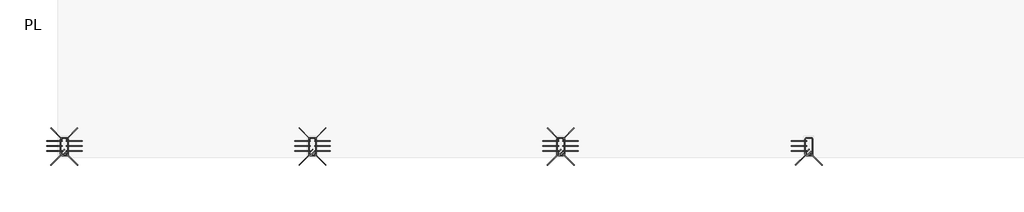
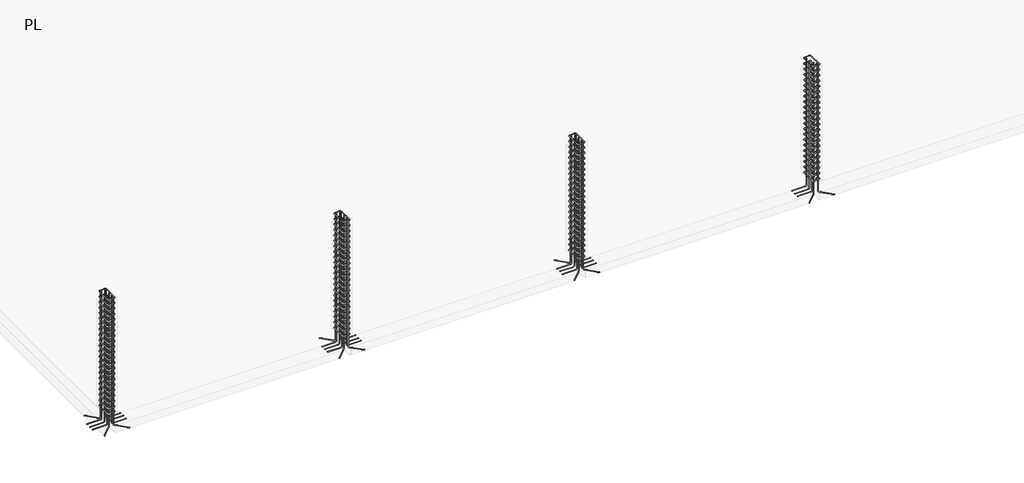
# One storey, part 3 of 10: 25 reinforcing bars.
"""IFC4 building model written with IfcOpenShell, lengths in millimetres."""

from ifc_helpers import new_model, si_unit, point, frame, origin, place, context, project, spatial, polyline, circle_curve, trimmed, segment, composite_curve, source, transform, mapped, element, save
from ifc_brep_helpers import swept_disk

model = new_model("IFC4")

# Units and contexts
model_context = context("Model", 3, world=origin())
ifc_project = project(units=[si_unit("LENGTHUNIT", "METRE", prefix="MILLI")], contexts=[model_context])

# Site, building, storey
site = spatial("IfcSite", under=ifc_project)
building = spatial("IfcBuilding", under=site)
storey = spatial("IfcBuildingStorey", under=building, Name="PL", Elevation=271.0)

# Reinforcing bars
placement = place(None, origin())
reinforcing_bar_shape = source(origin(), model_context, "Body", "SolidModel", [
    swept_disk(composite_curve([segment(polyline([(-16703.4864005, -20354.2223078, 301.0), (-16791.1676414, -20441.9035486, 301.0)]), True, "CONTINUOUS"), segment(trimmed(circle_curve(frame((-16769.9544379, -20463.1167521, 301.0), z_axis=(0.0, 0.0, 1.0), x_axis=(-21.21320349999951, 21.21320349999951, 0.0)), 30.0), [point((-16791.1676414, -20441.9035486, 301.0))], [point((-16769.9544379, -20493.1167521, 301.0))], True, "CARTESIAN"), True, "CONTINUOUS"), segment(polyline([(-16769.9544379, -20493.1167521, 301.0), (-16651.9544379, -20493.1167521, 301.0)]), True, "CONTINUOUS"), segment(trimmed(circle_curve(frame((-16651.9544379, -20463.1167521, 301.0), z_axis=(0.0, 0.0, 1.0), x_axis=(0.0, -30.0, 0.0)), 30.0), [point((-16651.9544379, -20493.1167521, 301.0))], [point((-16621.9544379, -20463.1167521, 301.0))], True, "CARTESIAN"), True, "CONTINUOUS"), segment(polyline([(-16621.9544379, -20463.1167521, 301.0), (-16621.9544379, -20095.1167521, 301.0)]), True, "CONTINUOUS"), segment(trimmed(circle_curve(frame((-16651.8864962, -20095.1167521, 298.9821084), z_axis=(-0.06726305234213417, 0.0, 0.9977352764083365), x_axis=(29.93205830000079, 0.0, 2.0178915999999845)), 30.0), [point((-16621.9544379, -20095.1167521, 301.0))], [point((-16651.8864962, -20065.1167521, 298.9821084))], True, "CARTESIAN"), True, "CONTINUOUS"), segment(polyline([(-16651.8864962, -20065.1167521, 298.9821084), (-16770.0223796, -20065.1167521, 291.0178916)]), True, "CONTINUOUS"), segment(trimmed(circle_curve(frame((-16770.0223796, -20095.1167521, 291.0178916), z_axis=(-0.06726305234213417, 0.0, 0.9977352764083365), x_axis=(0.0, 30.0, 0.0)), 30.0), [point((-16770.0223796, -20065.1167521, 291.0178916))], [point((-16799.9544379, -20095.1167521, 289.0))], True, "CARTESIAN"), True, "CONTINUOUS"), segment(polyline([(-16799.9544379, -20095.1167521, 289.0), (-16799.9544379, -20463.1167521, 289.0)]), True, "CONTINUOUS"), segment(trimmed(circle_curve(frame((-16769.9544379, -20463.1167521, 289.0), z_axis=(0.0, 0.0, 1.0), x_axis=(-30.0, 0.0, 0.0)), 30.0), [point((-16799.9544379, -20463.1167521, 289.0))], [point((-16748.7412345, -20484.3299555, 289.0))], True, "CARTESIAN"), True, "CONTINUOUS"), segment(polyline([(-16748.7412345, -20484.3299555, 289.0), (-16661.0599936, -20396.6487146, 289.0)]), True, "CONTINUOUS")], self_intersect=False), 6.0),
])
element("IfcReinforcingBar", 1, at=placement, inside=storey, context=model_context, shape_type="MappedRepresentation", body=[
    mapped(reinforcing_bar_shape, transform((0.0, 0.0, 0.0), x_axis=(1.0, 0.0, 0.0), y_axis=(0.0, 1.0, 0.0), z_axis=(0.0, 0.0, 1.0))),
    mapped(reinforcing_bar_shape, transform((0.0, 0.0, 149.2571429), x_axis=(1.0, 0.0, 0.0), y_axis=(0.0, 1.0, 0.0), z_axis=(0.0, 0.0, 1.0))),
    mapped(reinforcing_bar_shape, transform((0.0, 0.0, 298.5142857), x_axis=(1.0, 0.0, 0.0), y_axis=(0.0, 1.0, 0.0), z_axis=(0.0, 0.0, 1.0))),
    mapped(reinforcing_bar_shape, transform((0.0, 0.0, 447.7714286), x_axis=(1.0, 0.0, 0.0), y_axis=(0.0, 1.0, 0.0), z_axis=(0.0, 0.0, 1.0))),
    mapped(reinforcing_bar_shape, transform((0.0, 0.0, 597.0285714), x_axis=(1.0, 0.0, 0.0), y_axis=(0.0, 1.0, 0.0), z_axis=(0.0, 0.0, 1.0))),
    mapped(reinforcing_bar_shape, transform((0.0, 0.0, 746.2857143), x_axis=(1.0, 0.0, 0.0), y_axis=(0.0, 1.0, 0.0), z_axis=(0.0, 0.0, 1.0))),
    mapped(reinforcing_bar_shape, transform((0.0, 0.0, 895.5428571), x_axis=(1.0, 0.0, 0.0), y_axis=(0.0, 1.0, 0.0), z_axis=(0.0, 0.0, 1.0))),
    mapped(reinforcing_bar_shape, transform((0.0, 0.0, 1044.8), x_axis=(1.0, 0.0, 0.0), y_axis=(0.0, 1.0, 0.0), z_axis=(0.0, 0.0, 1.0))),
    mapped(reinforcing_bar_shape, transform((0.0, 0.0, 1194.0571429), x_axis=(1.0, 0.0, 0.0), y_axis=(0.0, 1.0, 0.0), z_axis=(0.0, 0.0, 1.0))),
    mapped(reinforcing_bar_shape, transform((0.0, 0.0, 1343.3142857), x_axis=(1.0, 0.0, 0.0), y_axis=(0.0, 1.0, 0.0), z_axis=(0.0, 0.0, 1.0))),
    mapped(reinforcing_bar_shape, transform((0.0, 0.0, 1492.5714286), x_axis=(1.0, 0.0, 0.0), y_axis=(0.0, 1.0, 0.0), z_axis=(0.0, 0.0, 1.0))),
    mapped(reinforcing_bar_shape, transform((0.0, 0.0, 1641.8285714), x_axis=(1.0, 0.0, 0.0), y_axis=(0.0, 1.0, 0.0), z_axis=(0.0, 0.0, 1.0))),
    mapped(reinforcing_bar_shape, transform((0.0, 0.0, 1791.0857143), x_axis=(1.0, 0.0, 0.0), y_axis=(0.0, 1.0, 0.0), z_axis=(0.0, 0.0, 1.0))),
    mapped(reinforcing_bar_shape, transform((0.0, 0.0, 1940.3428571), x_axis=(1.0, 0.0, 0.0), y_axis=(0.0, 1.0, 0.0), z_axis=(0.0, 0.0, 1.0))),
    mapped(reinforcing_bar_shape, transform((0.0, 0.0, 2089.6), x_axis=(1.0, 0.0, 0.0), y_axis=(0.0, 1.0, 0.0), z_axis=(0.0, 0.0, 1.0))),
    mapped(reinforcing_bar_shape, transform((0.0, 0.0, 2238.8571429), x_axis=(1.0, 0.0, 0.0), y_axis=(0.0, 1.0, 0.0), z_axis=(0.0, 0.0, 1.0))),
    mapped(reinforcing_bar_shape, transform((0.0, 0.0, 2388.1142857), x_axis=(1.0, 0.0, 0.0), y_axis=(0.0, 1.0, 0.0), z_axis=(0.0, 0.0, 1.0))),
    mapped(reinforcing_bar_shape, transform((0.0, 0.0, 2537.3714286), x_axis=(1.0, 0.0, 0.0), y_axis=(0.0, 1.0, 0.0), z_axis=(0.0, 0.0, 1.0))),
    mapped(reinforcing_bar_shape, transform((0.0, 0.0, 2686.6285714), x_axis=(1.0, 0.0, 0.0), y_axis=(0.0, 1.0, 0.0), z_axis=(0.0, 0.0, 1.0))),
    mapped(reinforcing_bar_shape, transform((0.0, 0.0, 2835.8857143), x_axis=(1.0, 0.0, 0.0), y_axis=(0.0, 1.0, 0.0), z_axis=(0.0, 0.0, 1.0))),
    mapped(reinforcing_bar_shape, transform((0.0, 0.0, 2985.1428571), x_axis=(1.0, 0.0, 0.0), y_axis=(0.0, 1.0, 0.0), z_axis=(0.0, 0.0, 1.0))),
    mapped(reinforcing_bar_shape, transform((0.0, 0.0, 3134.4), x_axis=(1.0, 0.0, 0.0), y_axis=(0.0, 1.0, 0.0), z_axis=(0.0, 0.0, 1.0))),
])
element("IfcReinforcingBar", 2, at=placement, inside=storey, context=model_context, shape_type="SolidModel", body=[
    swept_disk(composite_curve([segment(polyline([(-16768.0642232, -20464.0642439, 3441.4), (-16768.0642232, -20464.0642439, -35.0)]), True, "CONTINUOUS"), segment(trimmed(circle_curve(frame((-16789.2774266, -20485.2774473, -35.0), z_axis=(-0.7071067811865187, 0.7071067811865764, 0.0), x_axis=(21.213203400002385, 21.213203399998747, 0.0)), 30.0), [point((-16768.0642232, -20464.0642439, -35.0))], [point((-16789.2774266, -20485.2774473, -65.0))], True, "CARTESIAN"), True, "CONTINUOUS"), segment(polyline([(-16789.2774266, -20485.2774473, -65.0), (-17036.7648, -20732.7648207, -65.0)]), True, "CONTINUOUS")], self_intersect=False), 6.0),
])
element("IfcReinforcingBar", 3, at=placement, inside=storey, context=model_context, shape_type="SolidModel", body=[
    swept_disk(composite_curve([segment(polyline([(-16768.0642232, -20094.1692603, 3441.4), (-16768.0642232, -20094.1692603, -35.0)]), True, "CONTINUOUS"), segment(trimmed(circle_curve(frame((-16789.2774266, -20072.9560568, -35.0), z_axis=(0.7071067811865218, 0.7071067811865733, 0.0), x_axis=(21.213203400002385, -21.21320349999951, 0.0)), 30.0), [point((-16768.0642232, -20094.1692603, -35.0))], [point((-16789.2774266, -20072.9560568, -65.0))], True, "CARTESIAN"), True, "CONTINUOUS"), segment(polyline([(-16789.2774266, -20072.9560568, -65.0), (-17036.7648, -19825.4686834, -65.0)]), True, "CONTINUOUS")], self_intersect=False), 6.0),
])
element("IfcReinforcingBar", 4, at=placement, inside=storey, context=model_context, shape_type="SolidModel", body=[
    swept_disk(composite_curve([segment(polyline([(-16653.8446527, -20464.0642439, 3441.4), (-16653.8446527, -20464.0642439, -35.0)]), True, "CONTINUOUS"), segment(trimmed(circle_curve(frame((-16632.6314492, -20485.2774473, -35.0), z_axis=(-0.7071067811865248, -0.7071067811865703, 0.0), x_axis=(-21.213203500003146, 21.213203399998747, 0.0)), 30.0), [point((-16653.8446527, -20464.0642439, -35.0))], [point((-16632.6314492, -20485.2774473, -65.0))], True, "CARTESIAN"), True, "CONTINUOUS"), segment(polyline([(-16632.6314492, -20485.2774473, -65.0), (-16385.1440758, -20732.7648207, -65.0)]), True, "CONTINUOUS")], self_intersect=False), 6.0),
])
element("IfcReinforcingBar", 5, at=placement, inside=storey, context=model_context, shape_type="SolidModel", body=[
    swept_disk(composite_curve([segment(polyline([(-16653.8446527, -20094.1692603, 3441.4), (-16653.8446527, -20094.1692603, -35.0)]), True, "CONTINUOUS"), segment(trimmed(circle_curve(frame((-16632.6314492, -20072.9560568, -35.0), z_axis=(0.7071067811865157, -0.7071067811865794, 0.0), x_axis=(-21.213203500003146, -21.21320349999951, 0.0)), 30.0), [point((-16653.8446527, -20094.1692603, -35.0))], [point((-16632.6314492, -20072.9560568, -65.0))], True, "CARTESIAN"), True, "CONTINUOUS"), segment(polyline([(-16632.6314492, -20072.9560568, -65.0), (-16385.1440758, -19825.4686834, -65.0)]), True, "CONTINUOUS")], self_intersect=False), 6.0),
])
reinforcing_bar_2_shape = source(origin(), model_context, "Body", "SolidModel", [
    swept_disk(composite_curve([segment(polyline([(-16768.0642232, -20386.9117405, 3441.4), (-16768.0642232, -20386.9117405, -35.0)]), True, "CONTINUOUS"), segment(trimmed(circle_curve(frame((-16798.0642232, -20386.9117405, -35.0), z_axis=(0.0, 1.0, 0.0), x_axis=(30.0, 0.0, 0.0)), 30.0), [point((-16768.0642232, -20386.9117405, -35.0))], [point((-16798.0642232, -20386.9117405, -65.0))], True, "CARTESIAN"), True, "CONTINUOUS"), segment(polyline([(-16798.0642232, -20386.9117405, -65.0), (-17148.0642232, -20386.9117405, -65.0)]), True, "CONTINUOUS")], self_intersect=False), 6.0),
])
element("IfcReinforcingBar", 6, at=placement, inside=storey, context=model_context, shape_type="MappedRepresentation", body=[
    mapped(reinforcing_bar_2_shape, transform((0.0, 0.0, 0.0), x_axis=(1.0, 0.0, 0.0), y_axis=(0.0, 1.0, 0.0), z_axis=(0.0, 0.0, 1.0))),
    mapped(reinforcing_bar_2_shape, transform((0.0, 123.5823926, 0.0), x_axis=(1.0, 0.0, 0.0), y_axis=(0.0, 1.0, 0.0), z_axis=(0.0, 0.0, 1.0))),
    mapped(reinforcing_bar_2_shape, transform((0.0, 247.1647853, 0.0), x_axis=(1.0, 0.0, 0.0), y_axis=(0.0, 1.0, 0.0), z_axis=(0.0, 0.0, 1.0))),
])
reinforcing_bar_3_shape = source(origin(), model_context, "Body", "SolidModel", [
    swept_disk(composite_curve([segment(polyline([(-16653.8446527, -20386.9117405, 3441.4), (-16653.8446527, -20386.9117405, -35.0)]), True, "CONTINUOUS"), segment(trimmed(circle_curve(frame((-16623.8446527, -20386.9117405, -35.0), z_axis=(0.0, -1.0, 0.0), x_axis=(-30.0, 0.0, 0.0)), 30.0), [point((-16653.8446527, -20386.9117405, -35.0))], [point((-16623.8446527, -20386.9117405, -65.0))], True, "CARTESIAN"), True, "CONTINUOUS"), segment(polyline([(-16623.8446527, -20386.9117405, -65.0), (-16273.8446527, -20386.9117405, -65.0)]), True, "CONTINUOUS")], self_intersect=False), 6.0),
])
element("IfcReinforcingBar", 7, at=placement, inside=storey, context=model_context, shape_type="MappedRepresentation", body=[
    mapped(reinforcing_bar_3_shape, transform((0.0, 0.0, 0.0), x_axis=(1.0, 0.0, 0.0), y_axis=(0.0, 1.0, 0.0), z_axis=(0.0, 0.0, 1.0))),
    mapped(reinforcing_bar_3_shape, transform((0.0, 123.5823926, 0.0), x_axis=(1.0, 0.0, 0.0), y_axis=(0.0, 1.0, 0.0), z_axis=(0.0, 0.0, 1.0))),
    mapped(reinforcing_bar_3_shape, transform((0.0, 247.1647853, 0.0), x_axis=(1.0, 0.0, 0.0), y_axis=(0.0, 1.0, 0.0), z_axis=(0.0, 0.0, 1.0))),
])
reinforcing_bar_4_shape = source(origin(), model_context, "Body", "SolidModel", [
    swept_disk(composite_curve([segment(polyline([(-22799.4864005, -20354.2223078, 301.0), (-22887.1676414, -20441.9035486, 301.0)]), True, "CONTINUOUS"), segment(trimmed(circle_curve(frame((-22865.9544379, -20463.1167521, 301.0), z_axis=(0.0, 0.0, 1.0), x_axis=(-21.21320349999951, 21.21320349999951, 0.0)), 30.0), [point((-22887.1676414, -20441.9035486, 301.0))], [point((-22865.9544379, -20493.1167521, 301.0))], True, "CARTESIAN"), True, "CONTINUOUS"), segment(polyline([(-22865.9544379, -20493.1167521, 301.0), (-22747.9544379, -20493.1167521, 301.0)]), True, "CONTINUOUS"), segment(trimmed(circle_curve(frame((-22747.9544379, -20463.1167521, 301.0), z_axis=(0.0, 0.0, 1.0), x_axis=(0.0, -30.0, 0.0)), 30.0), [point((-22747.9544379, -20493.1167521, 301.0))], [point((-22717.9544379, -20463.1167521, 301.0))], True, "CARTESIAN"), True, "CONTINUOUS"), segment(polyline([(-22717.9544379, -20463.1167521, 301.0), (-22717.9544379, -20095.1167521, 301.0)]), True, "CONTINUOUS"), segment(trimmed(circle_curve(frame((-22747.8864962, -20095.1167521, 298.9821084), z_axis=(-0.06726305234213417, 0.0, 0.9977352764083365), x_axis=(29.93205830000079, 0.0, 2.0178915999999845)), 30.0), [point((-22717.9544379, -20095.1167521, 301.0))], [point((-22747.8864962, -20065.1167521, 298.9821084))], True, "CARTESIAN"), True, "CONTINUOUS"), segment(polyline([(-22747.8864962, -20065.1167521, 298.9821084), (-22866.0223796, -20065.1167521, 291.0178916)]), True, "CONTINUOUS"), segment(trimmed(circle_curve(frame((-22866.0223796, -20095.1167521, 291.0178916), z_axis=(-0.06726305234213417, 0.0, 0.9977352764083365), x_axis=(0.0, 30.0, 0.0)), 30.0), [point((-22866.0223796, -20065.1167521, 291.0178916))], [point((-22895.9544379, -20095.1167521, 289.0))], True, "CARTESIAN"), True, "CONTINUOUS"), segment(polyline([(-22895.9544379, -20095.1167521, 289.0), (-22895.9544379, -20463.1167521, 289.0)]), True, "CONTINUOUS"), segment(trimmed(circle_curve(frame((-22865.9544379, -20463.1167521, 289.0), z_axis=(0.0, 0.0, 1.0), x_axis=(-30.0, 0.0, 0.0)), 30.0), [point((-22895.9544379, -20463.1167521, 289.0))], [point((-22844.7412345, -20484.3299555, 289.0))], True, "CARTESIAN"), True, "CONTINUOUS"), segment(polyline([(-22844.7412345, -20484.3299555, 289.0), (-22757.0599936, -20396.6487146, 289.0)]), True, "CONTINUOUS")], self_intersect=False), 6.0),
])
element("IfcReinforcingBar", 8, at=placement, inside=storey, context=model_context, shape_type="MappedRepresentation", body=[
    mapped(reinforcing_bar_4_shape, transform((0.0, 0.0, 0.0), x_axis=(1.0, 0.0, 0.0), y_axis=(0.0, 1.0, 0.0), z_axis=(0.0, 0.0, 1.0))),
    mapped(reinforcing_bar_4_shape, transform((0.0, 0.0, 149.2571429), x_axis=(1.0, 0.0, 0.0), y_axis=(0.0, 1.0, 0.0), z_axis=(0.0, 0.0, 1.0))),
    mapped(reinforcing_bar_4_shape, transform((0.0, 0.0, 298.5142857), x_axis=(1.0, 0.0, 0.0), y_axis=(0.0, 1.0, 0.0), z_axis=(0.0, 0.0, 1.0))),
    mapped(reinforcing_bar_4_shape, transform((0.0, 0.0, 447.7714286), x_axis=(1.0, 0.0, 0.0), y_axis=(0.0, 1.0, 0.0), z_axis=(0.0, 0.0, 1.0))),
    mapped(reinforcing_bar_4_shape, transform((0.0, 0.0, 597.0285714), x_axis=(1.0, 0.0, 0.0), y_axis=(0.0, 1.0, 0.0), z_axis=(0.0, 0.0, 1.0))),
    mapped(reinforcing_bar_4_shape, transform((0.0, 0.0, 746.2857143), x_axis=(1.0, 0.0, 0.0), y_axis=(0.0, 1.0, 0.0), z_axis=(0.0, 0.0, 1.0))),
    mapped(reinforcing_bar_4_shape, transform((0.0, 0.0, 895.5428571), x_axis=(1.0, 0.0, 0.0), y_axis=(0.0, 1.0, 0.0), z_axis=(0.0, 0.0, 1.0))),
    mapped(reinforcing_bar_4_shape, transform((0.0, 0.0, 1044.8), x_axis=(1.0, 0.0, 0.0), y_axis=(0.0, 1.0, 0.0), z_axis=(0.0, 0.0, 1.0))),
    mapped(reinforcing_bar_4_shape, transform((0.0, 0.0, 1194.0571429), x_axis=(1.0, 0.0, 0.0), y_axis=(0.0, 1.0, 0.0), z_axis=(0.0, 0.0, 1.0))),
    mapped(reinforcing_bar_4_shape, transform((0.0, 0.0, 1343.3142857), x_axis=(1.0, 0.0, 0.0), y_axis=(0.0, 1.0, 0.0), z_axis=(0.0, 0.0, 1.0))),
    mapped(reinforcing_bar_4_shape, transform((0.0, 0.0, 1492.5714286), x_axis=(1.0, 0.0, 0.0), y_axis=(0.0, 1.0, 0.0), z_axis=(0.0, 0.0, 1.0))),
    mapped(reinforcing_bar_4_shape, transform((0.0, 0.0, 1641.8285714), x_axis=(1.0, 0.0, 0.0), y_axis=(0.0, 1.0, 0.0), z_axis=(0.0, 0.0, 1.0))),
    mapped(reinforcing_bar_4_shape, transform((0.0, 0.0, 1791.0857143), x_axis=(1.0, 0.0, 0.0), y_axis=(0.0, 1.0, 0.0), z_axis=(0.0, 0.0, 1.0))),
    mapped(reinforcing_bar_4_shape, transform((0.0, 0.0, 1940.3428571), x_axis=(1.0, 0.0, 0.0), y_axis=(0.0, 1.0, 0.0), z_axis=(0.0, 0.0, 1.0))),
    mapped(reinforcing_bar_4_shape, transform((0.0, 0.0, 2089.6), x_axis=(1.0, 0.0, 0.0), y_axis=(0.0, 1.0, 0.0), z_axis=(0.0, 0.0, 1.0))),
    mapped(reinforcing_bar_4_shape, transform((0.0, 0.0, 2238.8571429), x_axis=(1.0, 0.0, 0.0), y_axis=(0.0, 1.0, 0.0), z_axis=(0.0, 0.0, 1.0))),
    mapped(reinforcing_bar_4_shape, transform((0.0, 0.0, 2388.1142857), x_axis=(1.0, 0.0, 0.0), y_axis=(0.0, 1.0, 0.0), z_axis=(0.0, 0.0, 1.0))),
    mapped(reinforcing_bar_4_shape, transform((0.0, 0.0, 2537.3714286), x_axis=(1.0, 0.0, 0.0), y_axis=(0.0, 1.0, 0.0), z_axis=(0.0, 0.0, 1.0))),
    mapped(reinforcing_bar_4_shape, transform((0.0, 0.0, 2686.6285714), x_axis=(1.0, 0.0, 0.0), y_axis=(0.0, 1.0, 0.0), z_axis=(0.0, 0.0, 1.0))),
    mapped(reinforcing_bar_4_shape, transform((0.0, 0.0, 2835.8857143), x_axis=(1.0, 0.0, 0.0), y_axis=(0.0, 1.0, 0.0), z_axis=(0.0, 0.0, 1.0))),
    mapped(reinforcing_bar_4_shape, transform((0.0, 0.0, 2985.1428571), x_axis=(1.0, 0.0, 0.0), y_axis=(0.0, 1.0, 0.0), z_axis=(0.0, 0.0, 1.0))),
    mapped(reinforcing_bar_4_shape, transform((0.0, 0.0, 3134.4), x_axis=(1.0, 0.0, 0.0), y_axis=(0.0, 1.0, 0.0), z_axis=(0.0, 0.0, 1.0))),
])
element("IfcReinforcingBar", 9, at=placement, inside=storey, context=model_context, shape_type="SolidModel", body=[
    swept_disk(composite_curve([segment(polyline([(-22864.0642232, -20464.0642439, 3441.4), (-22864.0642232, -20464.0642439, -35.0)]), True, "CONTINUOUS"), segment(trimmed(circle_curve(frame((-22885.2774266, -20485.2774473, -35.0), z_axis=(-0.7071067811865187, 0.7071067811865764, 0.0), x_axis=(21.213203400002385, 21.213203399998747, 0.0)), 30.0), [point((-22864.0642232, -20464.0642439, -35.0))], [point((-22885.2774266, -20485.2774473, -65.0))], True, "CARTESIAN"), True, "CONTINUOUS"), segment(polyline([(-22885.2774266, -20485.2774473, -65.0), (-23132.7648, -20732.7648207, -65.0)]), True, "CONTINUOUS")], self_intersect=False), 6.0),
])
element("IfcReinforcingBar", 10, at=placement, inside=storey, context=model_context, shape_type="SolidModel", body=[
    swept_disk(composite_curve([segment(polyline([(-22864.0642232, -20094.1692603, 3441.4), (-22864.0642232, -20094.1692603, -35.0)]), True, "CONTINUOUS"), segment(trimmed(circle_curve(frame((-22885.2774266, -20072.9560568, -35.0), z_axis=(0.7071067811865218, 0.7071067811865733, 0.0), x_axis=(21.213203400002385, -21.21320349999951, 0.0)), 30.0), [point((-22864.0642232, -20094.1692603, -35.0))], [point((-22885.2774266, -20072.9560568, -65.0))], True, "CARTESIAN"), True, "CONTINUOUS"), segment(polyline([(-22885.2774266, -20072.9560568, -65.0), (-23132.7648, -19825.4686834, -65.0)]), True, "CONTINUOUS")], self_intersect=False), 6.0),
])
element("IfcReinforcingBar", 11, at=placement, inside=storey, context=model_context, shape_type="SolidModel", body=[
    swept_disk(composite_curve([segment(polyline([(-22749.8446527, -20464.0642439, 3441.4), (-22749.8446527, -20464.0642439, -35.0)]), True, "CONTINUOUS"), segment(trimmed(circle_curve(frame((-22728.6314492, -20485.2774473, -35.0), z_axis=(-0.7071067811865248, -0.7071067811865703, 0.0), x_axis=(-21.213203500003146, 21.213203399998747, 0.0)), 30.0), [point((-22749.8446527, -20464.0642439, -35.0))], [point((-22728.6314492, -20485.2774473, -65.0))], True, "CARTESIAN"), True, "CONTINUOUS"), segment(polyline([(-22728.6314492, -20485.2774473, -65.0), (-22481.1440758, -20732.7648207, -65.0)]), True, "CONTINUOUS")], self_intersect=False), 6.0),
])
element("IfcReinforcingBar", 12, at=placement, inside=storey, context=model_context, shape_type="SolidModel", body=[
    swept_disk(composite_curve([segment(polyline([(-22749.8446527, -20094.1692603, 3441.4), (-22749.8446527, -20094.1692603, -35.0)]), True, "CONTINUOUS"), segment(trimmed(circle_curve(frame((-22728.6314492, -20072.9560568, -35.0), z_axis=(0.7071067811865157, -0.7071067811865794, 0.0), x_axis=(-21.213203500003146, -21.21320349999951, 0.0)), 30.0), [point((-22749.8446527, -20094.1692603, -35.0))], [point((-22728.6314492, -20072.9560568, -65.0))], True, "CARTESIAN"), True, "CONTINUOUS"), segment(polyline([(-22728.6314492, -20072.9560568, -65.0), (-22481.1440758, -19825.4686834, -65.0)]), True, "CONTINUOUS")], self_intersect=False), 6.0),
])
reinforcing_bar_5_shape = source(origin(), model_context, "Body", "SolidModel", [
    swept_disk(composite_curve([segment(polyline([(-22864.0642232, -20386.9117405, 3441.4), (-22864.0642232, -20386.9117405, -35.0)]), True, "CONTINUOUS"), segment(trimmed(circle_curve(frame((-22894.0642232, -20386.9117405, -35.0), z_axis=(0.0, 1.0, 0.0), x_axis=(30.0, 0.0, 0.0)), 30.0), [point((-22864.0642232, -20386.9117405, -35.0))], [point((-22894.0642232, -20386.9117405, -65.0))], True, "CARTESIAN"), True, "CONTINUOUS"), segment(polyline([(-22894.0642232, -20386.9117405, -65.0), (-23244.0642232, -20386.9117405, -65.0)]), True, "CONTINUOUS")], self_intersect=False), 6.0),
])
element("IfcReinforcingBar", 13, at=placement, inside=storey, context=model_context, shape_type="MappedRepresentation", body=[
    mapped(reinforcing_bar_5_shape, transform((0.0, 0.0, 0.0), x_axis=(1.0, 0.0, 0.0), y_axis=(0.0, 1.0, 0.0), z_axis=(0.0, 0.0, 1.0))),
    mapped(reinforcing_bar_5_shape, transform((0.0, 123.5823926, 0.0), x_axis=(1.0, 0.0, 0.0), y_axis=(0.0, 1.0, 0.0), z_axis=(0.0, 0.0, 1.0))),
    mapped(reinforcing_bar_5_shape, transform((0.0, 247.1647853, 0.0), x_axis=(1.0, 0.0, 0.0), y_axis=(0.0, 1.0, 0.0), z_axis=(0.0, 0.0, 1.0))),
])
reinforcing_bar_6_shape = source(origin(), model_context, "Body", "SolidModel", [
    swept_disk(composite_curve([segment(polyline([(-22749.8446527, -20386.9117405, 3441.4), (-22749.8446527, -20386.9117405, -35.0)]), True, "CONTINUOUS"), segment(trimmed(circle_curve(frame((-22719.8446527, -20386.9117405, -35.0), z_axis=(0.0, -1.0, 0.0), x_axis=(-30.0, 0.0, 0.0)), 30.0), [point((-22749.8446527, -20386.9117405, -35.0))], [point((-22719.8446527, -20386.9117405, -65.0))], True, "CARTESIAN"), True, "CONTINUOUS"), segment(polyline([(-22719.8446527, -20386.9117405, -65.0), (-22369.8446527, -20386.9117405, -65.0)]), True, "CONTINUOUS")], self_intersect=False), 6.0),
])
element("IfcReinforcingBar", 14, at=placement, inside=storey, context=model_context, shape_type="MappedRepresentation", body=[
    mapped(reinforcing_bar_6_shape, transform((0.0, 0.0, 0.0), x_axis=(1.0, 0.0, 0.0), y_axis=(0.0, 1.0, 0.0), z_axis=(0.0, 0.0, 1.0))),
    mapped(reinforcing_bar_6_shape, transform((0.0, 123.5823926, 0.0), x_axis=(1.0, 0.0, 0.0), y_axis=(0.0, 1.0, 0.0), z_axis=(0.0, 0.0, 1.0))),
    mapped(reinforcing_bar_6_shape, transform((0.0, 247.1647853, 0.0), x_axis=(1.0, 0.0, 0.0), y_axis=(0.0, 1.0, 0.0), z_axis=(0.0, 0.0, 1.0))),
])
reinforcing_bar_7_shape = source(origin(), model_context, "Body", "SolidModel", [
    swept_disk(composite_curve([segment(polyline([(-10607.4864005, -20354.2223078, 301.0), (-10695.1676414, -20441.9035486, 301.0)]), True, "CONTINUOUS"), segment(trimmed(circle_curve(frame((-10673.9544379, -20463.1167521, 301.0), z_axis=(0.0, 0.0, 1.0), x_axis=(-21.21320349999951, 21.21320349999951, 0.0)), 30.0), [point((-10695.1676414, -20441.9035486, 301.0))], [point((-10673.9544379, -20493.1167521, 301.0))], True, "CARTESIAN"), True, "CONTINUOUS"), segment(polyline([(-10673.9544379, -20493.1167521, 301.0), (-10555.9544379, -20493.1167521, 301.0)]), True, "CONTINUOUS"), segment(trimmed(circle_curve(frame((-10555.9544379, -20463.1167521, 301.0), z_axis=(0.0, 0.0, 1.0), x_axis=(0.0, -30.0, 0.0)), 30.0), [point((-10555.9544379, -20493.1167521, 301.0))], [point((-10525.9544379, -20463.1167521, 301.0))], True, "CARTESIAN"), True, "CONTINUOUS"), segment(polyline([(-10525.9544379, -20463.1167521, 301.0), (-10525.9544379, -20095.1167521, 301.0)]), True, "CONTINUOUS"), segment(trimmed(circle_curve(frame((-10555.8864962, -20095.1167521, 298.9821084), z_axis=(-0.06726305234213417, 0.0, 0.9977352764083365), x_axis=(29.93205830000079, 0.0, 2.0178915999999845)), 30.0), [point((-10525.9544379, -20095.1167521, 301.0))], [point((-10555.8864962, -20065.1167521, 298.9821084))], True, "CARTESIAN"), True, "CONTINUOUS"), segment(polyline([(-10555.8864962, -20065.1167521, 298.9821084), (-10674.0223796, -20065.1167521, 291.0178916)]), True, "CONTINUOUS"), segment(trimmed(circle_curve(frame((-10674.0223796, -20095.1167521, 291.0178916), z_axis=(-0.06726305234213417, 0.0, 0.9977352764083365), x_axis=(0.0, 30.0, 0.0)), 30.0), [point((-10674.0223796, -20065.1167521, 291.0178916))], [point((-10703.9544379, -20095.1167521, 289.0))], True, "CARTESIAN"), True, "CONTINUOUS"), segment(polyline([(-10703.9544379, -20095.1167521, 289.0), (-10703.9544379, -20463.1167521, 289.0)]), True, "CONTINUOUS"), segment(trimmed(circle_curve(frame((-10673.9544379, -20463.1167521, 289.0), z_axis=(0.0, 0.0, 1.0), x_axis=(-30.0, 0.0, 0.0)), 30.0), [point((-10703.9544379, -20463.1167521, 289.0))], [point((-10652.7412345, -20484.3299555, 289.0))], True, "CARTESIAN"), True, "CONTINUOUS"), segment(polyline([(-10652.7412345, -20484.3299555, 289.0), (-10565.0599936, -20396.6487146, 289.0)]), True, "CONTINUOUS")], self_intersect=False), 6.0),
])
element("IfcReinforcingBar", 15, at=placement, inside=storey, context=model_context, shape_type="MappedRepresentation", body=[
    mapped(reinforcing_bar_7_shape, transform((0.0, 0.0, 0.0), x_axis=(1.0, 0.0, 0.0), y_axis=(0.0, 1.0, 0.0), z_axis=(0.0, 0.0, 1.0))),
    mapped(reinforcing_bar_7_shape, transform((0.0, 0.0, 149.2571429), x_axis=(1.0, 0.0, 0.0), y_axis=(0.0, 1.0, 0.0), z_axis=(0.0, 0.0, 1.0))),
    mapped(reinforcing_bar_7_shape, transform((0.0, 0.0, 298.5142857), x_axis=(1.0, 0.0, 0.0), y_axis=(0.0, 1.0, 0.0), z_axis=(0.0, 0.0, 1.0))),
    mapped(reinforcing_bar_7_shape, transform((0.0, 0.0, 447.7714286), x_axis=(1.0, 0.0, 0.0), y_axis=(0.0, 1.0, 0.0), z_axis=(0.0, 0.0, 1.0))),
    mapped(reinforcing_bar_7_shape, transform((0.0, 0.0, 597.0285714), x_axis=(1.0, 0.0, 0.0), y_axis=(0.0, 1.0, 0.0), z_axis=(0.0, 0.0, 1.0))),
    mapped(reinforcing_bar_7_shape, transform((0.0, 0.0, 746.2857143), x_axis=(1.0, 0.0, 0.0), y_axis=(0.0, 1.0, 0.0), z_axis=(0.0, 0.0, 1.0))),
    mapped(reinforcing_bar_7_shape, transform((0.0, 0.0, 895.5428571), x_axis=(1.0, 0.0, 0.0), y_axis=(0.0, 1.0, 0.0), z_axis=(0.0, 0.0, 1.0))),
    mapped(reinforcing_bar_7_shape, transform((0.0, 0.0, 1044.8), x_axis=(1.0, 0.0, 0.0), y_axis=(0.0, 1.0, 0.0), z_axis=(0.0, 0.0, 1.0))),
    mapped(reinforcing_bar_7_shape, transform((0.0, 0.0, 1194.0571429), x_axis=(1.0, 0.0, 0.0), y_axis=(0.0, 1.0, 0.0), z_axis=(0.0, 0.0, 1.0))),
    mapped(reinforcing_bar_7_shape, transform((0.0, 0.0, 1343.3142857), x_axis=(1.0, 0.0, 0.0), y_axis=(0.0, 1.0, 0.0), z_axis=(0.0, 0.0, 1.0))),
    mapped(reinforcing_bar_7_shape, transform((0.0, 0.0, 1492.5714286), x_axis=(1.0, 0.0, 0.0), y_axis=(0.0, 1.0, 0.0), z_axis=(0.0, 0.0, 1.0))),
    mapped(reinforcing_bar_7_shape, transform((0.0, 0.0, 1641.8285714), x_axis=(1.0, 0.0, 0.0), y_axis=(0.0, 1.0, 0.0), z_axis=(0.0, 0.0, 1.0))),
    mapped(reinforcing_bar_7_shape, transform((0.0, 0.0, 1791.0857143), x_axis=(1.0, 0.0, 0.0), y_axis=(0.0, 1.0, 0.0), z_axis=(0.0, 0.0, 1.0))),
    mapped(reinforcing_bar_7_shape, transform((0.0, 0.0, 1940.3428571), x_axis=(1.0, 0.0, 0.0), y_axis=(0.0, 1.0, 0.0), z_axis=(0.0, 0.0, 1.0))),
    mapped(reinforcing_bar_7_shape, transform((0.0, 0.0, 2089.6), x_axis=(1.0, 0.0, 0.0), y_axis=(0.0, 1.0, 0.0), z_axis=(0.0, 0.0, 1.0))),
    mapped(reinforcing_bar_7_shape, transform((0.0, 0.0, 2238.8571429), x_axis=(1.0, 0.0, 0.0), y_axis=(0.0, 1.0, 0.0), z_axis=(0.0, 0.0, 1.0))),
    mapped(reinforcing_bar_7_shape, transform((0.0, 0.0, 2388.1142857), x_axis=(1.0, 0.0, 0.0), y_axis=(0.0, 1.0, 0.0), z_axis=(0.0, 0.0, 1.0))),
    mapped(reinforcing_bar_7_shape, transform((0.0, 0.0, 2537.3714286), x_axis=(1.0, 0.0, 0.0), y_axis=(0.0, 1.0, 0.0), z_axis=(0.0, 0.0, 1.0))),
    mapped(reinforcing_bar_7_shape, transform((0.0, 0.0, 2686.6285714), x_axis=(1.0, 0.0, 0.0), y_axis=(0.0, 1.0, 0.0), z_axis=(0.0, 0.0, 1.0))),
    mapped(reinforcing_bar_7_shape, transform((0.0, 0.0, 2835.8857143), x_axis=(1.0, 0.0, 0.0), y_axis=(0.0, 1.0, 0.0), z_axis=(0.0, 0.0, 1.0))),
    mapped(reinforcing_bar_7_shape, transform((0.0, 0.0, 2985.1428571), x_axis=(1.0, 0.0, 0.0), y_axis=(0.0, 1.0, 0.0), z_axis=(0.0, 0.0, 1.0))),
    mapped(reinforcing_bar_7_shape, transform((0.0, 0.0, 3134.4), x_axis=(1.0, 0.0, 0.0), y_axis=(0.0, 1.0, 0.0), z_axis=(0.0, 0.0, 1.0))),
])
element("IfcReinforcingBar", 16, at=placement, inside=storey, context=model_context, shape_type="SolidModel", body=[
    swept_disk(composite_curve([segment(polyline([(-10672.0642232, -20464.0642439, 3441.4), (-10672.0642232, -20464.0642439, -35.0)]), True, "CONTINUOUS"), segment(trimmed(circle_curve(frame((-10693.2774266, -20485.2774473, -35.0), z_axis=(-0.7071067811865187, 0.7071067811865764, 0.0), x_axis=(21.213203400000566, 21.213203399998747, 0.0)), 30.0), [point((-10672.0642232, -20464.0642439, -35.0))], [point((-10693.2774266, -20485.2774473, -65.0))], True, "CARTESIAN"), True, "CONTINUOUS"), segment(polyline([(-10693.2774266, -20485.2774473, -65.0), (-10940.7648, -20732.7648207, -65.0)]), True, "CONTINUOUS")], self_intersect=False), 6.0),
])
element("IfcReinforcingBar", 17, at=placement, inside=storey, context=model_context, shape_type="SolidModel", body=[
    swept_disk(composite_curve([segment(polyline([(-10672.0642232, -20094.1692603, 3441.4), (-10672.0642232, -20094.1692603, -35.0)]), True, "CONTINUOUS"), segment(trimmed(circle_curve(frame((-10693.2774266, -20072.9560568, -35.0), z_axis=(0.7071067811865218, 0.7071067811865733, 0.0), x_axis=(21.213203400000566, -21.21320349999951, 0.0)), 30.0), [point((-10672.0642232, -20094.1692603, -35.0))], [point((-10693.2774266, -20072.9560568, -65.0))], True, "CARTESIAN"), True, "CONTINUOUS"), segment(polyline([(-10693.2774266, -20072.9560568, -65.0), (-10940.7648, -19825.4686834, -65.0)]), True, "CONTINUOUS")], self_intersect=False), 6.0),
])
element("IfcReinforcingBar", 18, at=placement, inside=storey, context=model_context, shape_type="SolidModel", body=[
    swept_disk(composite_curve([segment(polyline([(-10557.8446527, -20464.0642439, 3441.4), (-10557.8446527, -20464.0642439, -35.0)]), True, "CONTINUOUS"), segment(trimmed(circle_curve(frame((-10536.6314492, -20485.2774473, -35.0), z_axis=(-0.7071067811865248, -0.7071067811865703, 0.0), x_axis=(-21.21320349999951, 21.213203399998747, 0.0)), 30.0), [point((-10557.8446527, -20464.0642439, -35.0))], [point((-10536.6314492, -20485.2774473, -65.0))], True, "CARTESIAN"), True, "CONTINUOUS"), segment(polyline([(-10536.6314492, -20485.2774473, -65.0), (-10289.1440758, -20732.7648207, -65.0)]), True, "CONTINUOUS")], self_intersect=False), 6.0),
])
element("IfcReinforcingBar", 19, at=placement, inside=storey, context=model_context, shape_type="SolidModel", body=[
    swept_disk(composite_curve([segment(polyline([(-10557.8446527, -20094.1692603, 3441.4), (-10557.8446527, -20094.1692603, -35.0)]), True, "CONTINUOUS"), segment(trimmed(circle_curve(frame((-10536.6314492, -20072.9560568, -35.0), z_axis=(0.7071067811865157, -0.7071067811865794, 0.0), x_axis=(-21.21320349999951, -21.21320349999951, 0.0)), 30.0), [point((-10557.8446527, -20094.1692603, -35.0))], [point((-10536.6314492, -20072.9560568, -65.0))], True, "CARTESIAN"), True, "CONTINUOUS"), segment(polyline([(-10536.6314492, -20072.9560568, -65.0), (-10289.1440758, -19825.4686834, -65.0)]), True, "CONTINUOUS")], self_intersect=False), 6.0),
])
reinforcing_bar_8_shape = source(origin(), model_context, "Body", "SolidModel", [
    swept_disk(composite_curve([segment(polyline([(-10672.0642232, -20386.9117405, 3441.4), (-10672.0642232, -20386.9117405, -35.0)]), True, "CONTINUOUS"), segment(trimmed(circle_curve(frame((-10702.0642232, -20386.9117405, -35.0), z_axis=(0.0, 1.0, 0.0), x_axis=(30.0, 0.0, 0.0)), 30.0), [point((-10672.0642232, -20386.9117405, -35.0))], [point((-10702.0642232, -20386.9117405, -65.0))], True, "CARTESIAN"), True, "CONTINUOUS"), segment(polyline([(-10702.0642232, -20386.9117405, -65.0), (-11052.0642232, -20386.9117405, -65.0)]), True, "CONTINUOUS")], self_intersect=False), 6.0),
])
element("IfcReinforcingBar", 20, at=placement, inside=storey, context=model_context, shape_type="MappedRepresentation", body=[
    mapped(reinforcing_bar_8_shape, transform((0.0, 0.0, 0.0), x_axis=(1.0, 0.0, 0.0), y_axis=(0.0, 1.0, 0.0), z_axis=(0.0, 0.0, 1.0))),
    mapped(reinforcing_bar_8_shape, transform((0.0, 123.5823926, 0.0), x_axis=(1.0, 0.0, 0.0), y_axis=(0.0, 1.0, 0.0), z_axis=(0.0, 0.0, 1.0))),
    mapped(reinforcing_bar_8_shape, transform((0.0, 247.1647853, 0.0), x_axis=(1.0, 0.0, 0.0), y_axis=(0.0, 1.0, 0.0), z_axis=(0.0, 0.0, 1.0))),
])
reinforcing_bar_9_shape = source(origin(), model_context, "Body", "SolidModel", [
    swept_disk(composite_curve([segment(polyline([(-10557.8446527, -20386.9117405, 3441.4), (-10557.8446527, -20386.9117405, -35.0)]), True, "CONTINUOUS"), segment(trimmed(circle_curve(frame((-10527.8446527, -20386.9117405, -35.0), z_axis=(0.0, -1.0, 0.0), x_axis=(-30.0, 0.0, 0.0)), 30.0), [point((-10557.8446527, -20386.9117405, -35.0))], [point((-10527.8446527, -20386.9117405, -65.0))], True, "CARTESIAN"), True, "CONTINUOUS"), segment(polyline([(-10527.8446527, -20386.9117405, -65.0), (-10177.8446527, -20386.9117405, -65.0)]), True, "CONTINUOUS")], self_intersect=False), 6.0),
])
element("IfcReinforcingBar", 21, at=placement, inside=storey, context=model_context, shape_type="MappedRepresentation", body=[
    mapped(reinforcing_bar_9_shape, transform((0.0, 0.0, 0.0), x_axis=(1.0, 0.0, 0.0), y_axis=(0.0, 1.0, 0.0), z_axis=(0.0, 0.0, 1.0))),
    mapped(reinforcing_bar_9_shape, transform((0.0, 123.5823926, 0.0), x_axis=(1.0, 0.0, 0.0), y_axis=(0.0, 1.0, 0.0), z_axis=(0.0, 0.0, 1.0))),
    mapped(reinforcing_bar_9_shape, transform((0.0, 247.1647853, 0.0), x_axis=(1.0, 0.0, 0.0), y_axis=(0.0, 1.0, 0.0), z_axis=(0.0, 0.0, 1.0))),
])
reinforcing_bar_10_shape = source(origin(), model_context, "Body", "SolidModel", [
    swept_disk(composite_curve([segment(polyline([(-4511.4864005, -20354.2223078, 301.0), (-4599.1676414, -20441.9035486, 301.0)]), True, "CONTINUOUS"), segment(trimmed(circle_curve(frame((-4577.9544379, -20463.1167521, 301.0), z_axis=(0.0, 0.0, 1.0), x_axis=(-21.213203500000418, 21.21320349999951, 0.0)), 30.0), [point((-4599.1676414, -20441.9035486, 301.0))], [point((-4577.9544379, -20493.1167521, 301.0))], True, "CARTESIAN"), True, "CONTINUOUS"), segment(polyline([(-4577.9544379, -20493.1167521, 301.0), (-4459.9544379, -20493.1167521, 301.0)]), True, "CONTINUOUS"), segment(trimmed(circle_curve(frame((-4459.9544379, -20463.1167521, 301.0), z_axis=(0.0, 0.0, 1.0), x_axis=(0.0, -30.0, 0.0)), 30.0), [point((-4459.9544379, -20493.1167521, 301.0))], [point((-4429.9544379, -20463.1167521, 301.0))], True, "CARTESIAN"), True, "CONTINUOUS"), segment(polyline([(-4429.9544379, -20463.1167521, 301.0), (-4429.9544379, -20095.1167521, 301.0)]), True, "CONTINUOUS"), segment(trimmed(circle_curve(frame((-4459.8864962, -20095.1167521, 298.9821084), z_axis=(-0.06726305234213417, 0.0, 0.9977352764083365), x_axis=(29.93205829999988, 0.0, 2.0178915999999845)), 30.0), [point((-4429.9544379, -20095.1167521, 301.0))], [point((-4459.8864962, -20065.1167521, 298.9821084))], True, "CARTESIAN"), True, "CONTINUOUS"), segment(polyline([(-4459.8864962, -20065.1167521, 298.9821084), (-4578.0223796, -20065.1167521, 291.0178916)]), True, "CONTINUOUS"), segment(trimmed(circle_curve(frame((-4578.0223796, -20095.1167521, 291.0178916), z_axis=(-0.06726305234213417, 0.0, 0.9977352764083365), x_axis=(0.0, 30.0, 0.0)), 30.0), [point((-4578.0223796, -20065.1167521, 291.0178916))], [point((-4607.9544379, -20095.1167521, 289.0))], True, "CARTESIAN"), True, "CONTINUOUS"), segment(polyline([(-4607.9544379, -20095.1167521, 289.0), (-4607.9544379, -20463.1167521, 289.0)]), True, "CONTINUOUS"), segment(trimmed(circle_curve(frame((-4577.9544379, -20463.1167521, 289.0), z_axis=(0.0, 0.0, 1.0), x_axis=(-30.0, 0.0, 0.0)), 30.0), [point((-4607.9544379, -20463.1167521, 289.0))], [point((-4556.7412345, -20484.3299555, 289.0))], True, "CARTESIAN"), True, "CONTINUOUS"), segment(polyline([(-4556.7412345, -20484.3299555, 289.0), (-4469.0599936, -20396.6487146, 289.0)]), True, "CONTINUOUS")], self_intersect=False), 6.0),
])
element("IfcReinforcingBar", 22, at=placement, inside=storey, context=model_context, shape_type="MappedRepresentation", body=[
    mapped(reinforcing_bar_10_shape, transform((0.0, 0.0, 0.0), x_axis=(1.0, 0.0, 0.0), y_axis=(0.0, 1.0, 0.0), z_axis=(0.0, 0.0, 1.0))),
    mapped(reinforcing_bar_10_shape, transform((0.0, 0.0, 149.2571429), x_axis=(1.0, 0.0, 0.0), y_axis=(0.0, 1.0, 0.0), z_axis=(0.0, 0.0, 1.0))),
    mapped(reinforcing_bar_10_shape, transform((0.0, 0.0, 298.5142857), x_axis=(1.0, 0.0, 0.0), y_axis=(0.0, 1.0, 0.0), z_axis=(0.0, 0.0, 1.0))),
    mapped(reinforcing_bar_10_shape, transform((0.0, 0.0, 447.7714286), x_axis=(1.0, 0.0, 0.0), y_axis=(0.0, 1.0, 0.0), z_axis=(0.0, 0.0, 1.0))),
    mapped(reinforcing_bar_10_shape, transform((0.0, 0.0, 597.0285714), x_axis=(1.0, 0.0, 0.0), y_axis=(0.0, 1.0, 0.0), z_axis=(0.0, 0.0, 1.0))),
    mapped(reinforcing_bar_10_shape, transform((0.0, 0.0, 746.2857143), x_axis=(1.0, 0.0, 0.0), y_axis=(0.0, 1.0, 0.0), z_axis=(0.0, 0.0, 1.0))),
    mapped(reinforcing_bar_10_shape, transform((0.0, 0.0, 895.5428571), x_axis=(1.0, 0.0, 0.0), y_axis=(0.0, 1.0, 0.0), z_axis=(0.0, 0.0, 1.0))),
    mapped(reinforcing_bar_10_shape, transform((0.0, 0.0, 1044.8), x_axis=(1.0, 0.0, 0.0), y_axis=(0.0, 1.0, 0.0), z_axis=(0.0, 0.0, 1.0))),
    mapped(reinforcing_bar_10_shape, transform((0.0, 0.0, 1194.0571429), x_axis=(1.0, 0.0, 0.0), y_axis=(0.0, 1.0, 0.0), z_axis=(0.0, 0.0, 1.0))),
    mapped(reinforcing_bar_10_shape, transform((0.0, 0.0, 1343.3142857), x_axis=(1.0, 0.0, 0.0), y_axis=(0.0, 1.0, 0.0), z_axis=(0.0, 0.0, 1.0))),
    mapped(reinforcing_bar_10_shape, transform((0.0, 0.0, 1492.5714286), x_axis=(1.0, 0.0, 0.0), y_axis=(0.0, 1.0, 0.0), z_axis=(0.0, 0.0, 1.0))),
    mapped(reinforcing_bar_10_shape, transform((0.0, 0.0, 1641.8285714), x_axis=(1.0, 0.0, 0.0), y_axis=(0.0, 1.0, 0.0), z_axis=(0.0, 0.0, 1.0))),
    mapped(reinforcing_bar_10_shape, transform((0.0, 0.0, 1791.0857143), x_axis=(1.0, 0.0, 0.0), y_axis=(0.0, 1.0, 0.0), z_axis=(0.0, 0.0, 1.0))),
    mapped(reinforcing_bar_10_shape, transform((0.0, 0.0, 1940.3428571), x_axis=(1.0, 0.0, 0.0), y_axis=(0.0, 1.0, 0.0), z_axis=(0.0, 0.0, 1.0))),
    mapped(reinforcing_bar_10_shape, transform((0.0, 0.0, 2089.6), x_axis=(1.0, 0.0, 0.0), y_axis=(0.0, 1.0, 0.0), z_axis=(0.0, 0.0, 1.0))),
    mapped(reinforcing_bar_10_shape, transform((0.0, 0.0, 2238.8571429), x_axis=(1.0, 0.0, 0.0), y_axis=(0.0, 1.0, 0.0), z_axis=(0.0, 0.0, 1.0))),
    mapped(reinforcing_bar_10_shape, transform((0.0, 0.0, 2388.1142857), x_axis=(1.0, 0.0, 0.0), y_axis=(0.0, 1.0, 0.0), z_axis=(0.0, 0.0, 1.0))),
    mapped(reinforcing_bar_10_shape, transform((0.0, 0.0, 2537.3714286), x_axis=(1.0, 0.0, 0.0), y_axis=(0.0, 1.0, 0.0), z_axis=(0.0, 0.0, 1.0))),
    mapped(reinforcing_bar_10_shape, transform((0.0, 0.0, 2686.6285714), x_axis=(1.0, 0.0, 0.0), y_axis=(0.0, 1.0, 0.0), z_axis=(0.0, 0.0, 1.0))),
    mapped(reinforcing_bar_10_shape, transform((0.0, 0.0, 2835.8857143), x_axis=(1.0, 0.0, 0.0), y_axis=(0.0, 1.0, 0.0), z_axis=(0.0, 0.0, 1.0))),
    mapped(reinforcing_bar_10_shape, transform((0.0, 0.0, 2985.1428571), x_axis=(1.0, 0.0, 0.0), y_axis=(0.0, 1.0, 0.0), z_axis=(0.0, 0.0, 1.0))),
    mapped(reinforcing_bar_10_shape, transform((0.0, 0.0, 3134.4), x_axis=(1.0, 0.0, 0.0), y_axis=(0.0, 1.0, 0.0), z_axis=(0.0, 0.0, 1.0))),
])
element("IfcReinforcingBar", 23, at=placement, inside=storey, context=model_context, shape_type="SolidModel", body=[
    swept_disk(composite_curve([segment(polyline([(-4576.0642232, -20464.0642439, 3441.4), (-4576.0642232, -20464.0642439, -35.0)]), True, "CONTINUOUS"), segment(trimmed(circle_curve(frame((-4597.2774266, -20485.2774473, -35.0), z_axis=(-0.7071067811865187, 0.7071067811865764, 0.0), x_axis=(21.213203399999657, 21.213203399998747, 0.0)), 30.0), [point((-4576.0642232, -20464.0642439, -35.0))], [point((-4597.2774266, -20485.2774473, -65.0))], True, "CARTESIAN"), True, "CONTINUOUS"), segment(polyline([(-4597.2774266, -20485.2774473, -65.0), (-4844.7648, -20732.7648207, -65.0)]), True, "CONTINUOUS")], self_intersect=False), 6.0),
])
element("IfcReinforcingBar", 24, at=placement, inside=storey, context=model_context, shape_type="SolidModel", body=[
    swept_disk(composite_curve([segment(polyline([(-4461.8446527, -20464.0642439, 3441.4), (-4461.8446527, -20464.0642439, -35.0)]), True, "CONTINUOUS"), segment(trimmed(circle_curve(frame((-4440.6314492, -20485.2774473, -35.0), z_axis=(-0.7071067811865248, -0.7071067811865703, 0.0), x_axis=(-21.21320349999951, 21.213203399998747, 0.0)), 30.0), [point((-4461.8446527, -20464.0642439, -35.0))], [point((-4440.6314492, -20485.2774473, -65.0))], True, "CARTESIAN"), True, "CONTINUOUS"), segment(polyline([(-4440.6314492, -20485.2774473, -65.0), (-4193.1440758, -20732.7648207, -65.0)]), True, "CONTINUOUS")], self_intersect=False), 6.0),
])
reinforcing_bar_11_shape = source(origin(), model_context, "Body", "SolidModel", [
    swept_disk(composite_curve([segment(polyline([(-4576.0642232, -20386.9117405, 3441.4), (-4576.0642232, -20386.9117405, -35.0)]), True, "CONTINUOUS"), segment(trimmed(circle_curve(frame((-4606.0642232, -20386.9117405, -35.0), z_axis=(0.0, 1.0, 0.0), x_axis=(30.0, 0.0, 0.0)), 30.0), [point((-4576.0642232, -20386.9117405, -35.0))], [point((-4606.0642232, -20386.9117405, -65.0))], True, "CARTESIAN"), True, "CONTINUOUS"), segment(polyline([(-4606.0642232, -20386.9117405, -65.0), (-4956.0642232, -20386.9117405, -65.0)]), True, "CONTINUOUS")], self_intersect=False), 6.0),
])
element("IfcReinforcingBar", 25, at=placement, inside=storey, context=model_context, shape_type="MappedRepresentation", body=[
    mapped(reinforcing_bar_11_shape, transform((0.0, 0.0, 0.0), x_axis=(1.0, 0.0, 0.0), y_axis=(0.0, 1.0, 0.0), z_axis=(0.0, 0.0, 1.0))),
    mapped(reinforcing_bar_11_shape, transform((0.0, 123.5823926, 0.0), x_axis=(1.0, 0.0, 0.0), y_axis=(0.0, 1.0, 0.0), z_axis=(0.0, 0.0, 1.0))),
    mapped(reinforcing_bar_11_shape, transform((0.0, 247.1647853, 0.0), x_axis=(1.0, 0.0, 0.0), y_axis=(0.0, 1.0, 0.0), z_axis=(0.0, 0.0, 1.0))),
])

save(model, "model.ifc")

# Revit data of these elements
# Elements 1, 2, 3, 4, 5, 6, 7, 8, 9, 10, 11, 12, 13, 14, 15, 16, 17, 18, 19, 20, 21, 22, 23, 24, 25 (IfcReinforcingBar)
#   Phase Created = New Construction
